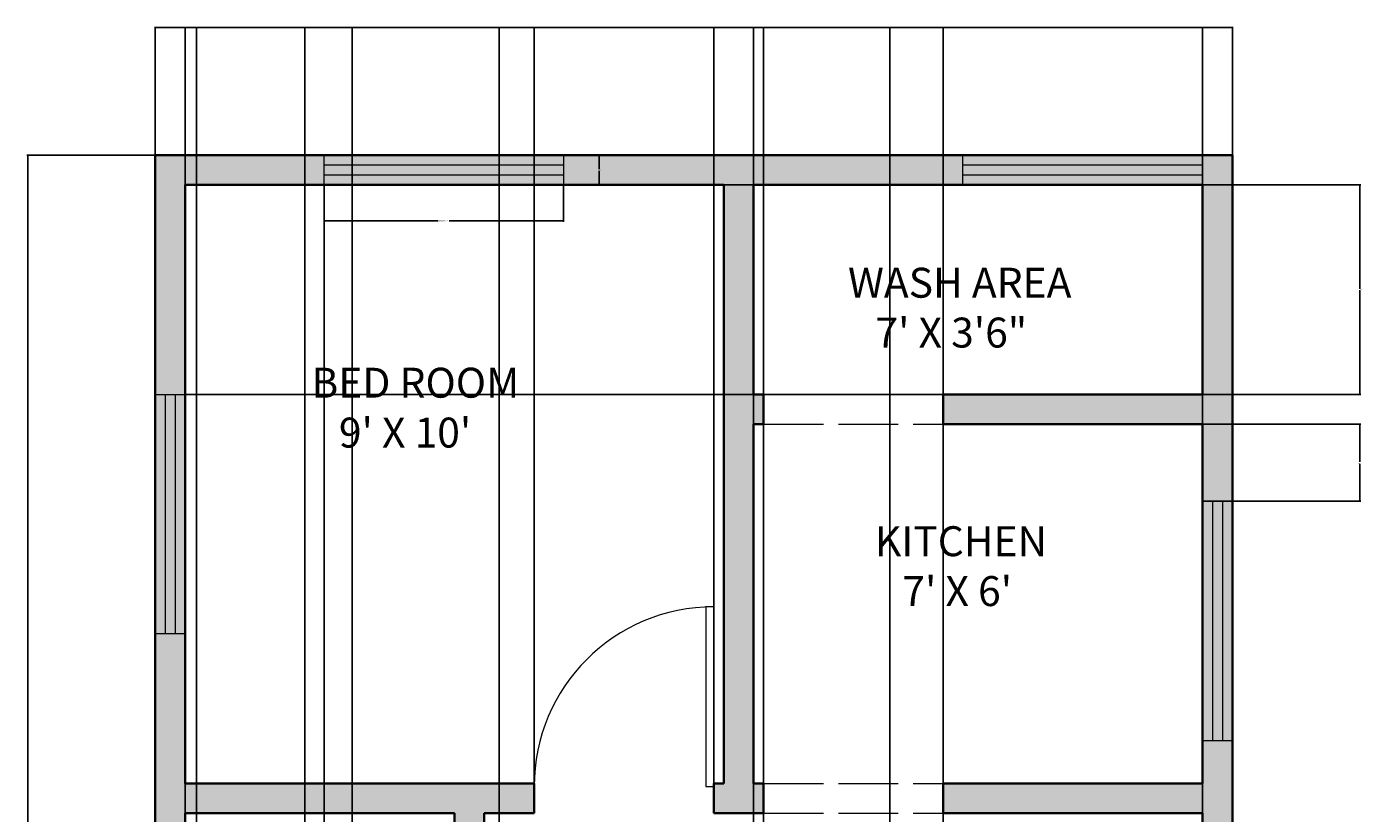
# Model space of a CAD drawing. Units: feet. Extents: x 4596233 to 4596501, y 5666486 to 5667044.
# Tile 3 of 3: x 4596233 to 4596501, y 5666886 to 5667044. Entities that reach past the tile are written whole.
import ezdxf

# ---------------------------------------------------------------- set-up
doc = ezdxf.new("R2010")
doc.units = ezdxf.units.FT
doc.linetypes.add('ACAD_ISO02W100', pattern=[15, 12, -3])
for name, color, linetype, lineweight in [('A-ANNO-DIMS', 2, 'Continuous', 18), ('A-DOOR-OVHD', 240, 'ACAD_ISO02W100', 18), ('A-WALL', 7, 'Continuous', 35), ('ANNOTATION', 170, 'Continuous', 18), ('DOOR', 240, 'Continuous', 18)]:
    doc.layers.add(name, color=color, linetype=linetype, lineweight=lineweight)
doc.layers.add('A-GLAZ', color=2, linetype='Continuous', lineweight=18, true_color=0xf1eb1f)
doc.layers.add('A-WALL-PATT', color=251, linetype='Continuous', lineweight=13, true_color=0x636466)
doc.styles.get("Standard").update_dxf_attribs({"font": 'arial.ttf'})
doc.dimstyles.get("Standard").update_dxf_attribs({"dimtxt": 0.18, "dimasz": 0.18, "dimexe": 0.18, "dimexo": 0.0625, "dimgap": 0.09, "dimtad": 0, "dimtih": 1, "dimtoh": 1, "dimdec": 0, "dimzin": 0, "dimdsep": 46, "dimlunit": 3, "dimtxsty": 'Standard', "dimcen": 0.09, "dimadec": 0, "dimazin": 0, "dimtfac": 1, "dimtdec": 0, "dimtofl": 0, "dimtmove": 0, "dimatfit": 3, "dimfxl": 1, "dimtolj": 1, "dimtzin": 0, "dimarcsym": 0})

# ---------------------------------------------------------------- blocks, each defined once
blk = doc.blocks.new('*U3')
for p, q in [((0, 0), (0, -6)), ((-40, 0), (-40, -6))]:
    blk.add_line(p, q)
blk.add_lwpolyline([(0, 0), (0, 40), (-1.75, 40), (-1.75, 0)], close=True)
blk.add_arc((0, 0), 40, 90, 180)
blk = doc.blocks.new('WIN-48IN')
h = blk.add_hatch(color=256)
h.dxf.hatch_style = 1
h.paths.add_polyline_path([(48, 2), (48, 4), (0, 4), (0, 2)])
for p, q in [((0, 6), (48, 6)), ((0, 0), (0, 6)), ((48, 6), (48, 0)), ((0, 4), (48, 4)), ((0, 2), (48, 2)), ((48, 0), (0, 0))]:
    blk.add_line(p, q)
blk = doc.blocks.new('*D7')
at = {"layer": 'A-ANNO-DIMS', "color": 0, "lineweight": -2, "transparency": 16777216}
for p, q in [((4596292.72, 5667012.09), (4596292.72, 5667004.77)), ((4596340.72, 5667012.09), (4596340.72, 5667004.77)), ((4596292.9, 5667004.95), (4596315.6, 5667004.95)), ((4596340.54, 5667004.95), (4596317.84, 5667004.95))]:
    blk.add_line(p, q, dxfattribs=at)
at = {"layer": 'A-ANNO-DIMS', "color": 0, "transparency": 16777216}
for points in [[(4596292.9, 5667004.98), (4596292.9, 5667004.92), (4596292.72, 5667004.95)], [(4596340.54, 5667004.98), (4596340.54, 5667004.92), (4596340.72, 5667004.95)]]:
    blk.add_solid(points, dxfattribs=at)
at = {"layer": 'Defpoints', "color": 0, "transparency": 16777216}
for p in [(4596292.72, 5667012.15), (4596340.72, 5667012.15), (4596340.72, 5667004.95)]:
    blk.add_point(p, dxfattribs=at)
at = {"layer": 'A-ANNO-DIMS', "color": 0, "transparency": 16777216, "insert": (4596316.72, 5667004.95), "char_height": 0.18, "attachment_point": 5}
blk.add_mtext('\\A1;WINDOW 48 TYP.', dxfattribs=at)
blk = doc.blocks.new('*D8')
at = {"layer": 'A-ANNO-DIMS', "color": 0, "lineweight": -2, "transparency": 16777216}
for p, q in [((4596340.78, 5667018.15), (4596348.1, 5667018.15)), ((4596347.92, 5667017.97), (4596347.92, 5667015.33)), ((4596347.92, 5667012.33), (4596347.92, 5667014.97)), ((4596340.78, 5667012.15), (4596348.1, 5667012.15))]:
    blk.add_line(p, q, dxfattribs=at)
at = {"layer": 'A-ANNO-DIMS', "color": 0, "transparency": 16777216}
for points in [[(4596347.89, 5667017.97), (4596347.95, 5667017.97), (4596347.92, 5667018.15)], [(4596347.89, 5667012.33), (4596347.95, 5667012.33), (4596347.92, 5667012.15)]]:
    blk.add_solid(points, dxfattribs=at)
at = {"layer": 'Defpoints', "color": 0, "transparency": 16777216}
for p in [(4596340.72, 5667018.15), (4596347.92, 5667018.15), (4596340.72, 5667012.15)]:
    blk.add_point(p, dxfattribs=at)
at = {"layer": 'A-ANNO-DIMS', "color": 0, "transparency": 16777216, "insert": (4596347.92, 5667015.15), "char_height": 0.18, "attachment_point": 5}
blk.add_mtext('\\A1;6 TYP.', dxfattribs=at)
blk = doc.blocks.new('*D11')
at = {"layer": 'A-ANNO-DIMS', "color": 0, "lineweight": -2, "transparency": 16777216}
for p, q in [((4596258.85, 5667018.21), (4596258.85, 5667043.88)), ((4596259.03, 5667043.7), (4596366.56, 5667043.7)), ((4596474.67, 5667043.7), (4596367.14, 5667043.7)), ((4596474.85, 5667018.21), (4596474.85, 5667043.88))]:
    blk.add_line(p, q, dxfattribs=at)
at = {"layer": 'A-ANNO-DIMS', "color": 0, "transparency": 16777216}
for points in [[(4596259.03, 5667043.73), (4596259.03, 5667043.67), (4596258.85, 5667043.7)], [(4596474.67, 5667043.73), (4596474.67, 5667043.67), (4596474.85, 5667043.7)]]:
    blk.add_solid(points, dxfattribs=at)
at = {"layer": 'Defpoints', "color": 0, "transparency": 16777216}
for p in [(4596474.85, 5667043.7), (4596258.85, 5667018.15), (4596474.85, 5667018.15)]:
    blk.add_point(p, dxfattribs=at)
at = {"layer": 'A-ANNO-DIMS', "color": 0, "transparency": 16777216, "insert": (4596366.85, 5667043.7), "char_height": 0.18, "attachment_point": 5}
blk.add_mtext('\\A1;216', dxfattribs=at)
blk = doc.blocks.new('*D12')
at = {"layer": 'A-ANNO-DIMS', "color": 0, "lineweight": -2, "transparency": 16777216}
for p, q in [((4596258.79, 5667018.15), (4596233.12, 5667018.15)), ((4596233.3, 5667017.97), (4596233.3, 5666784.33)), ((4596233.3, 5666550.33), (4596233.3, 5666783.97)), ((4596258.79, 5666550.15), (4596233.12, 5666550.15))]:
    blk.add_line(p, q, dxfattribs=at)
at = {"layer": 'A-ANNO-DIMS', "color": 0, "transparency": 16777216}
for points in [[(4596233.27, 5667017.97), (4596233.33, 5667017.97), (4596233.3, 5667018.15)], [(4596233.27, 5666550.33), (4596233.33, 5666550.33), (4596233.3, 5666550.15)]]:
    blk.add_solid(points, dxfattribs=at)
at = {"layer": 'Defpoints', "color": 0, "transparency": 16777216}
for p in [(4596233.3, 5667018.15), (4596258.85, 5667018.15), (4596258.85, 5666550.15)]:
    blk.add_point(p, dxfattribs=at)
at = {"layer": 'A-ANNO-DIMS', "color": 0, "transparency": 16777216, "insert": (4596233.3, 5666784.15), "char_height": 0.18, "attachment_point": 5}
blk.add_mtext('\\A1;468', dxfattribs=at)
blk = doc.blocks.new('*D15')
at = {"layer": 'A-ANNO-DIMS', "color": 0, "lineweight": -2, "transparency": 16777216}
for p, q in [((4596378.85, 5666964.09), (4596378.85, 5666485.84)), ((4596468.85, 5666964.09), (4596468.85, 5666485.84)), ((4596379.03, 5666486.02), (4596423.63, 5666486.02)), ((4596468.67, 5666486.02), (4596424.07, 5666486.02))]:
    blk.add_line(p, q, dxfattribs=at)
at = {"layer": 'A-ANNO-DIMS', "color": 0, "transparency": 16777216}
for points in [[(4596379.03, 5666486.05), (4596379.03, 5666485.99), (4596378.85, 5666486.02)], [(4596468.67, 5666486.05), (4596468.67, 5666485.99), (4596468.85, 5666486.02)]]:
    blk.add_solid(points, dxfattribs=at)
at = {"layer": 'Defpoints', "color": 0, "transparency": 16777216}
for p in [(4596378.85, 5666964.15), (4596468.85, 5666964.15), (4596468.85, 5666486.02)]:
    blk.add_point(p, dxfattribs=at)
at = {"layer": 'A-ANNO-DIMS', "color": 0, "transparency": 16777216, "insert": (4596423.85, 5666486.02), "char_height": 0.18, "attachment_point": 5}
blk.add_mtext('\\A1;90', dxfattribs=at)
blk = doc.blocks.new('*D17')
at = {"layer": 'A-ANNO-DIMS', "color": 0, "lineweight": -2, "transparency": 16777216}
for p, q in [((4596380.85, 5666688.21), (4596380.85, 5667043.88)), ((4596381.03, 5667043.7), (4596398.63, 5667043.7)), ((4596416.67, 5667043.7), (4596399.07, 5667043.7)), ((4596416.85, 5666688.21), (4596416.85, 5667043.88))]:
    blk.add_line(p, q, dxfattribs=at)
at = {"layer": 'A-ANNO-DIMS', "color": 0, "transparency": 16777216}
for points in [[(4596381.03, 5667043.73), (4596381.03, 5667043.67), (4596380.85, 5667043.7)], [(4596416.67, 5667043.73), (4596416.67, 5667043.67), (4596416.85, 5667043.7)]]:
    blk.add_solid(points, dxfattribs=at)
at = {"layer": 'Defpoints', "color": 0, "transparency": 16777216}
for p in [(4596416.85, 5667043.7), (4596380.85, 5666688.15), (4596416.85, 5666688.15)]:
    blk.add_point(p, dxfattribs=at)
at = {"layer": 'A-ANNO-DIMS', "color": 0, "transparency": 16777216, "insert": (4596398.85, 5667043.7), "char_height": 0.18, "attachment_point": 5}
blk.add_mtext('\\A1;36', dxfattribs=at)
blk = doc.blocks.new('*D20')
at = {"layer": 'A-ANNO-DIMS', "color": 0, "lineweight": -2, "transparency": 16777216}
for p, q in [((4596334.85, 5666892.21), (4596334.85, 5667043.88)), ((4596335.03, 5667043.7), (4596352.63, 5667043.7)), ((4596370.67, 5667043.7), (4596353.07, 5667043.7)), ((4596370.85, 5666892.21), (4596370.85, 5667043.88))]:
    blk.add_line(p, q, dxfattribs=at)
at = {"layer": 'A-ANNO-DIMS', "color": 0, "transparency": 16777216}
for points in [[(4596335.03, 5667043.73), (4596335.03, 5667043.67), (4596334.85, 5667043.7)], [(4596370.67, 5667043.73), (4596370.67, 5667043.67), (4596370.85, 5667043.7)]]:
    blk.add_solid(points, dxfattribs=at)
at = {"layer": 'Defpoints', "color": 0, "transparency": 16777216}
for p in [(4596370.85, 5667043.7), (4596334.85, 5666892.15), (4596370.85, 5666892.15)]:
    blk.add_point(p, dxfattribs=at)
at = {"layer": 'A-ANNO-DIMS', "color": 0, "transparency": 16777216, "insert": (4596352.85, 5667043.7), "char_height": 0.18, "attachment_point": 5}
blk.add_mtext('\\A1;36', dxfattribs=at)
blk = doc.blocks.new('*D22')
at = {"layer": 'A-ANNO-DIMS', "color": 0, "lineweight": -2, "transparency": 16777216}
for p, q in [((4596264.85, 5667012.09), (4596264.85, 5666485.84)), ((4596292.72, 5667012.09), (4596292.72, 5666485.84)), ((4596265.03, 5666486.02), (4596278.39, 5666486.02)), ((4596292.54, 5666486.02), (4596279.18, 5666486.02))]:
    blk.add_line(p, q, dxfattribs=at)
at = {"layer": 'A-ANNO-DIMS', "color": 0, "transparency": 16777216}
for points in [[(4596265.03, 5666486.05), (4596265.03, 5666485.99), (4596264.85, 5666486.02)], [(4596292.54, 5666486.05), (4596292.54, 5666485.99), (4596292.72, 5666486.02)]]:
    blk.add_solid(points, dxfattribs=at)
at = {"layer": 'Defpoints', "color": 0, "transparency": 16777216}
for p in [(4596264.85, 5667012.15), (4596292.72, 5667012.15), (4596292.72, 5666486.02)]:
    blk.add_point(p, dxfattribs=at)
at = {"layer": 'A-ANNO-DIMS', "color": 0, "transparency": 16777216, "insert": (4596278.78, 5666486.02), "char_height": 0.18, "attachment_point": 5}
blk.add_mtext('\\A1;27.87', dxfattribs=at)
blk = doc.blocks.new('*D23')
at = {"layer": 'A-ANNO-DIMS', "color": 0, "lineweight": -2, "transparency": 16777216}
for p, q in [((4596264.91, 5667012.15), (4596500.58, 5667012.15)), ((4596500.4, 5667011.97), (4596500.4, 5666991.32)), ((4596500.4, 5666970.3), (4596500.4, 5666990.95)), ((4596264.91, 5666970.12), (4596500.58, 5666970.12))]:
    blk.add_line(p, q, dxfattribs=at)
at = {"layer": 'A-ANNO-DIMS', "color": 0, "transparency": 16777216}
for points in [[(4596500.37, 5667011.97), (4596500.43, 5667011.97), (4596500.4, 5667012.15)], [(4596500.37, 5666970.3), (4596500.43, 5666970.3), (4596500.4, 5666970.12)]]:
    blk.add_solid(points, dxfattribs=at)
at = {"layer": 'Defpoints', "color": 0, "transparency": 16777216}
for p in [(4596264.85, 5667012.15), (4596500.4, 5667012.15), (4596264.85, 5666970.12)]:
    blk.add_point(p, dxfattribs=at)
at = {"layer": 'A-ANNO-DIMS', "color": 0, "transparency": 16777216, "insert": (4596500.4, 5666991.13), "char_height": 0.18, "attachment_point": 5}
blk.add_mtext('\\A1;42.03', dxfattribs=at)
blk = doc.blocks.new('*D24')
at = {"layer": 'A-ANNO-DIMS', "color": 0, "lineweight": -2, "transparency": 16777216}
for p, q in [((4596468.91, 5666964.15), (4596500.58, 5666964.15)), ((4596500.4, 5666963.97), (4596500.4, 5666956.61)), ((4596500.4, 5666948.89), (4596500.4, 5666956.25)), ((4596468.91, 5666948.71), (4596500.58, 5666948.71))]:
    blk.add_line(p, q, dxfattribs=at)
at = {"layer": 'A-ANNO-DIMS', "color": 0, "transparency": 16777216}
for points in [[(4596500.37, 5666963.97), (4596500.43, 5666963.97), (4596500.4, 5666964.15)], [(4596500.37, 5666948.89), (4596500.43, 5666948.89), (4596500.4, 5666948.71)]]:
    blk.add_solid(points, dxfattribs=at)
at = {"layer": 'Defpoints', "color": 0, "transparency": 16777216}
for p in [(4596468.85, 5666964.15), (4596468.85, 5666948.71), (4596500.4, 5666948.71)]:
    blk.add_point(p, dxfattribs=at)
at = {"layer": 'A-ANNO-DIMS', "color": 0, "transparency": 16777216, "insert": (4596500.4, 5666956.43), "char_height": 0.18, "attachment_point": 5}
blk.add_mtext('\\A1;15.44', dxfattribs=at)
blk = doc.blocks.new('*D28')
at = {"layer": 'A-ANNO-DIMS', "color": 0, "lineweight": -2, "transparency": 16777216}
for p, q in [((4596378.85, 5666556.21), (4596378.85, 5667043.88)), ((4596379.03, 5667043.7), (4596392.04, 5667043.7)), ((4596405.99, 5667043.7), (4596392.97, 5667043.7)), ((4596406.17, 5666556.21), (4596406.17, 5667043.88))]:
    blk.add_line(p, q, dxfattribs=at)
at = {"layer": 'A-ANNO-DIMS', "color": 0, "transparency": 16777216}
for points in [[(4596379.03, 5667043.73), (4596379.03, 5667043.67), (4596378.85, 5667043.7)], [(4596405.99, 5667043.73), (4596405.99, 5667043.67), (4596406.17, 5667043.7)]]:
    blk.add_solid(points, dxfattribs=at)
at = {"layer": 'Defpoints', "color": 0, "transparency": 16777216}
for p in [(4596406.17, 5667043.7), (4596378.85, 5666556.15), (4596406.17, 5666556.15)]:
    blk.add_point(p, dxfattribs=at)
at = {"layer": 'A-ANNO-DIMS', "color": 0, "transparency": 16777216, "insert": (4596392.51, 5667043.7), "char_height": 0.18, "attachment_point": 5}
blk.add_mtext('\\A1;27.317', dxfattribs=at)
blk = doc.blocks.new('*D33')
at = {"layer": 'A-ANNO-DIMS', "color": 0, "lineweight": -2, "transparency": 16777216}
for p, q in [((4596267.15, 5666650.02), (4596267.15, 5667043.88)), ((4596267.33, 5667043.7), (4596282.36, 5667043.7)), ((4596298.17, 5667043.7), (4596283.14, 5667043.7)), ((4596298.35, 5666650.02), (4596298.35, 5667043.88))]:
    blk.add_line(p, q, dxfattribs=at)
at = {"layer": 'A-ANNO-DIMS', "color": 0, "transparency": 16777216}
for points in [[(4596267.33, 5667043.73), (4596267.33, 5667043.67), (4596267.15, 5667043.7)], [(4596298.17, 5667043.73), (4596298.17, 5667043.67), (4596298.35, 5667043.7)]]:
    blk.add_solid(points, dxfattribs=at)
at = {"layer": 'Defpoints', "color": 0, "transparency": 16777216}
for p in [(4596298.35, 5667043.7), (4596267.15, 5666649.96), (4596298.35, 5666649.96)]:
    blk.add_point(p, dxfattribs=at)
at = {"layer": 'A-ANNO-DIMS', "color": 0, "transparency": 16777216, "insert": (4596282.75, 5667043.7), "char_height": 0.18, "attachment_point": 5}
blk.add_mtext('\\A1;31.19', dxfattribs=at)
blk = doc.blocks.new('*D34')
at = {"layer": 'A-ANNO-DIMS', "color": 0, "lineweight": -2, "transparency": 16777216}
for p, q in [((4596264.85, 5666892.21), (4596264.85, 5667043.88)), ((4596265.03, 5667043.7), (4596299.63, 5667043.7)), ((4596334.67, 5667043.7), (4596300.07, 5667043.7)), ((4596334.85, 5666892.21), (4596334.85, 5667043.88))]:
    blk.add_line(p, q, dxfattribs=at)
at = {"layer": 'A-ANNO-DIMS', "color": 0, "transparency": 16777216}
for points in [[(4596265.03, 5667043.73), (4596265.03, 5667043.67), (4596264.85, 5667043.7)], [(4596334.67, 5667043.73), (4596334.67, 5667043.67), (4596334.85, 5667043.7)]]:
    blk.add_solid(points, dxfattribs=at)
at = {"layer": 'Defpoints', "color": 0, "transparency": 16777216}
for p in [(4596334.85, 5667043.7), (4596264.85, 5666892.15), (4596334.85, 5666892.15)]:
    blk.add_point(p, dxfattribs=at)
at = {"layer": 'A-ANNO-DIMS', "color": 0, "transparency": 16777216, "insert": (4596299.85, 5667043.7), "char_height": 0.18, "attachment_point": 5}
blk.add_mtext('\\A1;70', dxfattribs=at)
blk = doc.blocks.new('*D35')
at = {"layer": 'A-ANNO-DIMS', "color": 0, "lineweight": -2, "transparency": 16777216}
for p, q in [((4596416.85, 5666688.21), (4596416.85, 5667043.88)), ((4596417.03, 5667043.7), (4596442.63, 5667043.7)), ((4596468.67, 5667043.7), (4596443.07, 5667043.7)), ((4596468.85, 5666688.21), (4596468.85, 5667043.88))]:
    blk.add_line(p, q, dxfattribs=at)
at = {"layer": 'A-ANNO-DIMS', "color": 0, "transparency": 16777216}
for points in [[(4596417.03, 5667043.73), (4596417.03, 5667043.67), (4596416.85, 5667043.7)], [(4596468.67, 5667043.73), (4596468.67, 5667043.67), (4596468.85, 5667043.7)]]:
    blk.add_solid(points, dxfattribs=at)
at = {"layer": 'Defpoints', "color": 0, "transparency": 16777216}
for p in [(4596468.85, 5667043.7), (4596416.85, 5666688.15), (4596468.85, 5666688.15)]:
    blk.add_point(p, dxfattribs=at)
at = {"layer": 'A-ANNO-DIMS', "color": 0, "transparency": 16777216, "insert": (4596442.85, 5667043.7), "char_height": 0.18, "attachment_point": 5}
blk.add_mtext('\\A1;52', dxfattribs=at)
blk = doc.blocks.new('*D37')
at = {"layer": 'A-ANNO-DIMS', "color": 0, "lineweight": -2, "transparency": 16777216}
for p, q in [((4596264.85, 5666688.21), (4596264.85, 5667043.88)), ((4596265.03, 5667043.7), (4596296.13, 5667043.7)), ((4596327.67, 5667043.7), (4596296.57, 5667043.7)), ((4596327.85, 5666688.21), (4596327.85, 5667043.88))]:
    blk.add_line(p, q, dxfattribs=at)
at = {"layer": 'A-ANNO-DIMS', "color": 0, "transparency": 16777216}
for points in [[(4596265.03, 5667043.73), (4596265.03, 5667043.67), (4596264.85, 5667043.7)], [(4596327.67, 5667043.73), (4596327.67, 5667043.67), (4596327.85, 5667043.7)]]:
    blk.add_solid(points, dxfattribs=at)
at = {"layer": 'Defpoints', "color": 0, "transparency": 16777216}
for p in [(4596327.85, 5667043.7), (4596264.85, 5666688.15), (4596327.85, 5666688.15)]:
    blk.add_point(p, dxfattribs=at)
at = {"layer": 'A-ANNO-DIMS', "color": 0, "transparency": 16777216, "insert": (4596296.35, 5667043.7), "char_height": 0.18, "attachment_point": 5}
blk.add_mtext('\\A1;63', dxfattribs=at)
blk = doc.blocks.new('*D39')
at = {"layer": 'A-ANNO-DIMS', "color": 0, "lineweight": -2, "transparency": 16777216}
for p, q in [((4596264.85, 5666760.21), (4596264.85, 5667043.88)), ((4596265.03, 5667043.7), (4596276.63, 5667043.7)), ((4596288.67, 5667043.7), (4596277.07, 5667043.7)), ((4596288.85, 5666760.21), (4596288.85, 5667043.88))]:
    blk.add_line(p, q, dxfattribs=at)
at = {"layer": 'A-ANNO-DIMS', "color": 0, "transparency": 16777216}
for points in [[(4596265.03, 5667043.73), (4596265.03, 5667043.67), (4596264.85, 5667043.7)], [(4596288.67, 5667043.73), (4596288.67, 5667043.67), (4596288.85, 5667043.7)]]:
    blk.add_solid(points, dxfattribs=at)
at = {"layer": 'Defpoints', "color": 0, "transparency": 16777216}
for p in [(4596288.85, 5667043.7), (4596264.85, 5666760.15), (4596288.85, 5666760.15)]:
    blk.add_point(p, dxfattribs=at)
at = {"layer": 'A-ANNO-DIMS', "color": 0, "transparency": 16777216, "insert": (4596276.85, 5667043.7), "char_height": 0.18, "attachment_point": 5}
blk.add_mtext('\\A1;24', dxfattribs=at)
blk = doc.blocks.new('*D43')
at = {"layer": 'A-ANNO-DIMS', "color": 0, "lineweight": -2, "transparency": 16777216}
for p, q in [((4596380.85, 5666970.21), (4596380.85, 5667043.88)), ((4596381.03, 5667043.7), (4596398.63, 5667043.7)), ((4596416.67, 5667043.7), (4596399.07, 5667043.7)), ((4596416.85, 5666970.21), (4596416.85, 5667043.88))]:
    blk.add_line(p, q, dxfattribs=at)
at = {"layer": 'A-ANNO-DIMS', "color": 0, "transparency": 16777216}
for points in [[(4596381.03, 5667043.73), (4596381.03, 5667043.67), (4596380.85, 5667043.7)], [(4596416.67, 5667043.73), (4596416.67, 5667043.67), (4596416.85, 5667043.7)]]:
    blk.add_solid(points, dxfattribs=at)
at = {"layer": 'Defpoints', "color": 0, "transparency": 16777216}
for p in [(4596416.85, 5667043.7), (4596380.85, 5666970.15), (4596416.85, 5666970.15)]:
    blk.add_point(p, dxfattribs=at)
at = {"layer": 'A-ANNO-DIMS', "color": 0, "transparency": 16777216, "insert": (4596398.85, 5667043.7), "char_height": 0.18, "attachment_point": 5}
blk.add_mtext('\\A1;36', dxfattribs=at)

msp = doc.modelspace()

# ---------------------------------------------------------------- hatches: boundary and pattern name
at = {"layer": 'A-WALL-PATT'}
h = msp.add_hatch(color=256, dxfattribs=at)
h.dxf.hatch_style = 1
h.paths.add_polyline_path([(4596474.8511, 5667018.1479), (4596258.8511, 5667018.1479), (4596258.8511, 5666550.1479), (4596474.8511, 5666550.1479)])
h.paths.add_polyline_path([(4596372.8511, 5667012.1479), (4596372.8511, 5666892.1479), (4596370.8511, 5666892.1479), (4596370.8511, 5666891.5479), (4596370.8511, 5666886.1479), (4596380.8511, 5666886.1479), (4596380.8511, 5666892.1479), (4596378.8511, 5666892.1479), (4596378.8511, 5666964.1479), (4596380.8511, 5666964.1479), (4596380.8511, 5666970.1479), (4596378.8511, 5666970.1479), (4596378.8511, 5667012.1479), (4596468.8511, 5667012.1479), (4596468.8511, 5666970.1479), (4596416.8511, 5666970.1479), (4596416.8511, 5666964.1479), (4596468.8511, 5666964.1479), (4596468.8511, 5666892.1479), (4596416.8511, 5666892.1479), (4596416.8511, 5666886.1479), (4596468.8511, 5666886.1479), (4596468.8511, 5666688.1479), (4596416.8511, 5666688.1479), (4596416.8511, 5666682.1479), (4596468.8511, 5666682.1479), (4596468.8511, 5666556.1479), (4596378.8511, 5666556.1479), (4596378.8511, 5666682.1479), (4596380.8511, 5666682.1479), (4596380.8511, 5666687.5479), (4596380.8511, 5666688.1479), (4596369.8511, 5666688.1479), (4596369.8511, 5666685.2979), (4596369.8511, 5666682.1479), (4596372.8511, 5666682.1479), (4596372.8511, 5666556.1479), (4596264.8511, 5666556.1479), (4596264.8511, 5666682.1479), (4596327.8511, 5666682.1479), (4596327.8511, 5666685.2979), (4596327.8511, 5666688.1479), (4596324.8511, 5666688.1479), (4596324.8511, 5666772.1479), (4596318.8511, 5666772.1479), (4596318.8511, 5666760.1479), (4596318.8511, 5666754.1479), (4596318.8511, 5666724.1479), (4596318.8511, 5666688.1479), (4596264.8511, 5666688.1479), (4596264.8511, 5666754.1479), (4596288.8511, 5666754.1479), (4596288.8511, 5666758.6479), (4596288.8511, 5666760.1479), (4596264.8511, 5666760.1479), (4596264.8511, 5666814.1479), (4596288.8511, 5666814.1479), (4596288.8511, 5666818.6479), (4596288.8511, 5666820.1479), (4596264.8511, 5666820.1479), (4596264.8511, 5666886.1479), (4596318.8511, 5666886.1479), (4596318.8511, 5666820.1479), (4596318.8511, 5666818.6479), (4596318.8511, 5666814.1479), (4596318.8511, 5666802.1479), (4596324.8511, 5666802.1479), (4596324.8511, 5666886.1479), (4596334.8511, 5666886.1479), (4596334.8511, 5666891.5479), (4596334.8511, 5666892.1479), (4596264.8511, 5666892.1479), (4596264.8511, 5667012.1479)], flags=16)
h.paths.add_polyline_path([(4596316.6338, 5666680.1479), (4596316.6338, 5666661.9608), (4596301.036, 5666661.9608), (4596301.036, 5666589.119), (4596370.916, 5666589.119), (4596370.916, 5666558.119), (4596267.1547, 5666558.119), (4596267.1547, 5666680.1479)], flags=0)
h.paths.add_polyline_path([(4596282.7503, 5666649.9608), (4596298.3459, 5666649.9608), (4596298.3459, 5666586.4128), (4596333.2108, 5666586.4128), (4596333.2108, 5666572.6335), (4596282.7503, 5666572.6335)], flags=0)
h.paths.add_polyline_path([(4596380.8511, 5666682.1479), (4596382.4261, 5666682.1479), (4596382.4261, 5666646.1479), (4596380.8511, 5666646.1479)], flags=0)
h.paths.add_polyline_path([(4596270.4341, 5666856.9819), (4596311.4805, 5666856.9819), (4596311.4805, 5666879.3708), (4596270.4341, 5666879.3708)], flags=8)
h.paths.add_polyline_path([(4596271.3283, 5666778.1649), (4596312.3747, 5666778.1649), (4596312.3747, 5666800.5538), (4596271.3283, 5666800.5538)], flags=8)
h.paths.add_polyline_path([(4596401.0723, 5666924.3036), (4596440.8622, 5666924.3036), (4596440.8622, 5666946.6925), (4596401.0723, 5666946.6925)], flags=8)
h.paths.add_polyline_path([(4596396.1839, 5666976.1395), (4596449.4963, 5666976.1395), (4596449.4963, 5666998.5283), (4596396.1839, 5666998.5283)], flags=8)
h.paths.add_polyline_path([(4596288.0879, 5666956.0844), (4596336.7264, 5666956.0844), (4596336.7264, 5666978.4732), (4596288.0879, 5666978.4732)], flags=8)
h.paths.add_polyline_path([(4596267.7433, 5666702.4027), (4596308.7897, 5666702.4027), (4596308.7897, 5666724.7916), (4596267.7433, 5666724.7916)], flags=8)
h.paths.add_polyline_path([(4596371.4978, 5666770.3665), (4596425.2768, 5666770.3665), (4596425.2768, 5666792.7553), (4596371.4978, 5666792.7553)], flags=8)
h.paths.add_polyline_path([(4596414.2198, 5666615.8536), (4596452.2908, 5666615.8536), (4596452.2908, 5666638.2424), (4596414.2198, 5666638.2424)], flags=8)
h.paths.add_polyline_path([(4596310.1554, 5666620.3865), (4596350.8825, 5666620.3865), (4596350.8825, 5666642.7753), (4596310.1554, 5666642.7753)], flags=8)
h = msp.add_hatch(color=256, dxfattribs=at)
h.dxf.hatch_style = 1
h.paths.add_polyline_path([(4596474.8511, 5667018.1479), (4596258.8511, 5667018.1479), (4596258.8511, 5666550.1479), (4596474.8511, 5666550.1479)])
h.paths.add_polyline_path([(4596468.8511, 5666970.1479), (4596416.8511, 5666970.1479), (4596416.8511, 5666964.1479), (4596468.8511, 5666964.1479), (4596468.8511, 5666892.1479), (4596416.8511, 5666892.1479), (4596416.8511, 5666886.1479), (4596468.8511, 5666886.1479), (4596468.8511, 5666688.1479), (4596416.8511, 5666688.1479), (4596416.8511, 5666682.1479), (4596468.8511, 5666682.1479), (4596468.8511, 5666556.1479), (4596378.8511, 5666556.1479), (4596378.8511, 5666682.1479), (4596380.8511, 5666682.1479), (4596380.8511, 5666687.5479), (4596380.8511, 5666688.1479), (4596369.8511, 5666688.1479), (4596369.8511, 5666685.2979), (4596369.8511, 5666682.1479), (4596372.8511, 5666682.1479), (4596372.8511, 5666556.1479), (4596264.8511, 5666556.1479), (4596264.8511, 5666682.1479), (4596327.8511, 5666682.1479), (4596327.8511, 5666685.2979), (4596327.8511, 5666688.1479), (4596324.8511, 5666688.1479), (4596324.8511, 5666772.1479), (4596318.8511, 5666772.1479), (4596318.8511, 5666760.1479), (4596318.8511, 5666754.1479), (4596318.8511, 5666724.1479), (4596318.8511, 5666688.1479), (4596264.8511, 5666688.1479), (4596264.8511, 5666754.1479), (4596288.8511, 5666754.1479), (4596288.8511, 5666758.6479), (4596288.8511, 5666760.1479), (4596264.8511, 5666760.1479), (4596264.8511, 5666814.1479), (4596288.8511, 5666814.1479), (4596288.8511, 5666818.6479), (4596288.8511, 5666820.1479), (4596264.8511, 5666820.1479), (4596264.8511, 5666886.1479), (4596318.8511, 5666886.1479), (4596318.8511, 5666820.1479), (4596318.8511, 5666818.6479), (4596318.8511, 5666814.1479), (4596318.8511, 5666802.1479), (4596324.8511, 5666802.1479), (4596324.8511, 5666886.1479), (4596334.8511, 5666886.1479), (4596334.8511, 5666891.5479), (4596334.8511, 5666892.1479), (4596264.8511, 5666892.1479), (4596264.8511, 5667012.1479), (4596372.8511, 5667012.1479), (4596372.8511, 5666892.1479), (4596370.8511, 5666892.1479), (4596370.8511, 5666891.5479), (4596370.8511, 5666886.1479), (4596380.8511, 5666886.1479), (4596380.8511, 5666892.1479), (4596378.8511, 5666892.1479), (4596378.8511, 5666964.1479), (4596380.8511, 5666964.1479), (4596380.8511, 5666970.1479), (4596378.8511, 5666970.1479), (4596378.8511, 5667012.1479), (4596468.8511, 5667012.1479)], flags=16)
h.paths.add_polyline_path([(4596382.4261, 5666646.1479), (4596380.8511, 5666646.1479), (4596380.8511, 5666682.1479), (4596382.4261, 5666682.1479)], flags=0)
h.paths.add_polyline_path([(4596316.6338, 5666680.1479), (4596316.6338, 5666661.9608), (4596301.036, 5666661.9608), (4596301.036, 5666589.119), (4596370.916, 5666589.119), (4596370.916, 5666558.119), (4596267.1547, 5666558.119), (4596267.1547, 5666680.1479)], flags=0)
h.paths.add_polyline_path([(4596282.7503, 5666649.9608), (4596298.3459, 5666649.9608), (4596298.3459, 5666586.4128), (4596333.2108, 5666586.4128), (4596333.2108, 5666572.6335), (4596282.7503, 5666572.6335)], flags=0)
h.paths.add_polyline_path([(4596270.4341, 5666856.9819), (4596311.4805, 5666856.9819), (4596311.4805, 5666879.3708), (4596270.4341, 5666879.3708)], flags=8)
h.paths.add_polyline_path([(4596271.3283, 5666778.1649), (4596312.3747, 5666778.1649), (4596312.3747, 5666800.5538), (4596271.3283, 5666800.5538)], flags=8)
h.paths.add_polyline_path([(4596401.0723, 5666924.3036), (4596440.8622, 5666924.3036), (4596440.8622, 5666946.6925), (4596401.0723, 5666946.6925)], flags=8)
h.paths.add_polyline_path([(4596396.1839, 5666976.1395), (4596449.4963, 5666976.1395), (4596449.4963, 5666998.5283), (4596396.1839, 5666998.5283)], flags=8)
h.paths.add_polyline_path([(4596288.0879, 5666956.0844), (4596336.7264, 5666956.0844), (4596336.7264, 5666978.4732), (4596288.0879, 5666978.4732)], flags=8)
h.paths.add_polyline_path([(4596267.7433, 5666702.4027), (4596308.7897, 5666702.4027), (4596308.7897, 5666724.7916), (4596267.7433, 5666724.7916)], flags=8)
h.paths.add_polyline_path([(4596371.4978, 5666770.3665), (4596425.2768, 5666770.3665), (4596425.2768, 5666792.7553), (4596371.4978, 5666792.7553)], flags=8)
h.paths.add_polyline_path([(4596414.2198, 5666615.8536), (4596452.2908, 5666615.8536), (4596452.2908, 5666638.2424), (4596414.2198, 5666638.2424)], flags=8)
h.paths.add_polyline_path([(4596310.1554, 5666620.3865), (4596350.8825, 5666620.3865), (4596350.8825, 5666642.7753), (4596310.1554, 5666642.7753)], flags=8)

# ---------------------------------------------------------------- linework, layer by layer
at = {"layer": 'A-DOOR-OVHD'}
for p, q in [((4596380.8511, 5666970.1479), (4596416.8511, 5666970.1479)), ((4596380.8511, 5666964.1479), (4596416.8511, 5666964.1479)), ((4596380.8511, 5666892.1479), (4596416.8511, 5666892.1479)), ((4596380.8511, 5666886.1479), (4596416.8511, 5666886.1479))]:
    msp.add_line(p, q, dxfattribs=at)
at = {"layer": 'A-WALL'}
for p, q in [((4596258.8511, 5667018.1479), (4596474.8511, 5667018.1479)), ((4596258.8511, 5666550.1479), (4596258.8511, 5667018.1479)), ((4596474.8511, 5667018.1479), (4596474.8511, 5666550.1479)), ((4596264.8511, 5667012.1479), (4596372.8511, 5667012.1479)), ((4596264.8511, 5666892.1479), (4596264.8511, 5667012.1479)), ((4596372.8511, 5666892.1479), (4596372.8511, 5667012.1479)), ((4596378.8511, 5667012.1479), (4596468.8511, 5667012.1479)), ((4596378.8511, 5666970.1479), (4596378.8511, 5667012.1479)), ((4596468.8511, 5667012.1479), (4596468.8511, 5666970.1479)), ((4596378.8511, 5666970.1479), (4596380.8511, 5666970.1479)), ((4596380.8511, 5666970.1479), (4596380.8511, 5666964.1479)), ((4596416.8511, 5666970.1479), (4596416.8511, 5666964.1479)), ((4596416.8511, 5666970.1479), (4596468.8511, 5666970.1479)), ((4596378.8511, 5666964.1479), (4596380.8511, 5666964.1479)), ((4596378.8511, 5666892.1479), (4596378.8511, 5666964.1479)), ((4596416.8511, 5666964.1479), (4596468.8511, 5666964.1479)), ((4596468.8511, 5666964.1479), (4596468.8511, 5666892.1479)), ((4596264.8511, 5666892.1479), (4596334.8511, 5666892.1479)), ((4596334.8511, 5666892.1479), (4596334.8511, 5666886.1479)), ((4596370.8511, 5666892.1479), (4596370.8511, 5666886.1479)), ((4596370.8511, 5666892.1479), (4596372.8511, 5666892.1479)), ((4596378.8511, 5666892.1479), (4596380.8511, 5666892.1479)), ((4596380.8511, 5666892.1479), (4596380.8511, 5666886.1479)), ((4596416.8511, 5666892.1479), (4596416.8511, 5666886.1479)), ((4596416.8511, 5666892.1479), (4596468.8511, 5666892.1479)), ((4596264.8511, 5666886.1479), (4596318.8511, 5666886.1479)), ((4596264.8511, 5666820.1479), (4596264.8511, 5666886.1479)), ((4596318.8511, 5666820.1479), (4596318.8511, 5666886.1479)), ((4596324.8511, 5666886.1479), (4596334.8511, 5666886.1479)), ((4596324.8511, 5666802.1479), (4596324.8511, 5666886.1479)), ((4596370.8511, 5666886.1479), (4596380.8511, 5666886.1479)), ((4596416.8511, 5666886.1479), (4596468.8511, 5666886.1479)), ((4596468.8511, 5666886.1479), (4596468.8511, 5666688.1479))]:
    msp.add_line(p, q, dxfattribs=at)

# ---------------------------------------------------------------- block references
at = {"layer": 'A-GLAZ'}
for p in [(4596292.718, 5667012.148), (4596420.7753, 5667012.148)]:
    msp.add_blockref('WIN-48IN', p, dxfattribs=at)
for p, rotation in [((4596258.8512, 5666970.1206), 270.0000000038905), ((4596468.8512, 5666948.707), 270.0000000067078)]:
    msp.add_blockref('WIN-48IN', p, dxfattribs=dict(at, rotation=rotation))
at = {"layer": 'DOOR', "xscale": 0.9000000000838191, "yscale": 0.9000000000838191, "zscale": 0.9000000000838191}
msp.add_blockref('*U3', (4596370.8511, 5666891.5479), dxfattribs=at)

# ---------------------------------------------------------------- texts
at = {"layer": 'ANNOTATION', "char_height": 6, "attachment_point": 1}
for s, width, insert in [('WASH AREA\\P   7\' X 3\'6"', 50.67683, (4596397.7863, 5666995.5427)), ("BED ROOM\\P   9' X 10'", 52.338365, (4596290.2018, 5666975.4916)), ("KITCHEN\\P   7' X 6'", 41.538385, (4596403.1862, 5666943.7068))]:
    msp.add_mtext_dynamic_manual_height_columns(s, width=width, gutter_width=12.5, heights=[0], dxfattribs=dict(at, insert=insert))

# ---------------------------------------------------------------- dimensions: what is measured, and where the dimension line sits
at = {"layer": 'A-ANNO-DIMS'}
for base, p1, p2, override, picture, middle in [((4596474.8511, 5667043.6979), (4596258.8511, 5667018.1479), (4596474.8511, 5667018.1479), {"dimdec": 0, "dimlfac": 1, "dimrnd": 0, "dimzin": 0, "dimdsep": 46, "dimlunit": 2}, '*D11', (4596366.8511, 5667043.6979)), ((4596334.8511, 5667043.6979), (4596264.8511, 5666892.1479), (4596334.8511, 5666892.1479), {"dimdec": 0, "dimlfac": 1, "dimrnd": 0, "dimzin": 0, "dimdsep": 46, "dimlunit": 2}, '*D34', (4596299.8511, 5667043.6979)), ((4596327.8511, 5667043.6979), (4596264.8511, 5666688.1479), (4596327.8511, 5666688.1479), {"dimdec": 0, "dimlfac": 1, "dimrnd": 0, "dimzin": 0, "dimdsep": 46, "dimlunit": 2}, '*D37', (4596296.3511, 5667043.6979)), ((4596288.8511, 5667043.6979), (4596264.8511, 5666760.1479), (4596288.8511, 5666760.1479), {"dimdec": 0, "dimlfac": 1, "dimrnd": 0, "dimzin": 0, "dimdsep": 46, "dimlunit": 2}, '*D39', (4596276.8511, 5667043.6979)), ((4596298.3459, 5667043.6979), (4596267.1547, 5666649.9608), (4596298.3459, 5666649.9608), {"dimdec": 2, "dimlfac": 1, "dimrnd": 0, "dimzin": 0, "dimdsep": 46, "dimlunit": 2}, '*D33', (4596282.7503, 5667043.6979)), ((4596370.8511, 5667043.6979), (4596334.8511, 5666892.1479), (4596370.8511, 5666892.1479), {"dimdec": 0, "dimlfac": 1, "dimrnd": 0, "dimzin": 0, "dimdsep": 46, "dimlunit": 2}, '*D20', (4596352.8511, 5667043.6979)), ((4596406.1677, 5667043.6979), (4596378.8511, 5666556.1479), (4596406.1677, 5666556.1479), {"dimdec": 3, "dimlfac": 1, "dimrnd": 0, "dimzin": 0, "dimdsep": 46, "dimlunit": 2}, '*D28', (4596392.5094, 5667043.6979)), ((4596416.8511, 5667043.6979), (4596380.8511, 5666688.1479), (4596416.8511, 5666688.1479), {"dimdec": 0, "dimlfac": 1, "dimrnd": 0, "dimzin": 0, "dimdsep": 46, "dimlunit": 2}, '*D17', (4596398.8511, 5667043.6979)), ((4596416.8511, 5667043.6979), (4596380.8511, 5666970.1479), (4596416.8511, 5666970.1479), {"dimdec": 0, "dimlfac": 1, "dimrnd": 0, "dimzin": 0, "dimdsep": 46, "dimlunit": 2}, '*D43', (4596398.8511, 5667043.6979)), ((4596468.8511, 5667043.6979), (4596416.8511, 5666688.1479), (4596468.8511, 5666688.1479), {"dimdec": 0, "dimlfac": 1, "dimrnd": 0, "dimzin": 0, "dimdsep": 46, "dimlunit": 2}, '*D35', (4596442.8511, 5667043.6979)), ((4596292.7184, 5666486.0229), (4596264.8511, 5667012.1479), (4596292.7184, 5667012.1479), {"dimdec": 2, "dimlfac": 1, "dimrnd": 0, "dimzin": 0, "dimdsep": 46, "dimlunit": 2}, '*D22', (4596278.7847, 5666486.0229)), ((4596468.8511, 5666486.0229), (4596378.8511, 5666964.1479), (4596468.8511, 5666964.1479), {"dimdec": 0, "dimlfac": 1, "dimrnd": 0, "dimzin": 0, "dimdsep": 46, "dimlunit": 2}, '*D15', (4596423.8511, 5666486.0229))]:
    dim = msp.add_linear_dim(base=base, p1=p1, p2=p2, dimstyle='Standard', override=override, dxfattribs=at)
    dim.commit()
    dim.dimension.update_dxf_attribs({"geometry": picture, "text_midpoint": middle})
for base, p1, p2, override, picture, middle in [((4596233.3011, 5667018.1479), (4596258.8511, 5666550.1479), (4596258.8511, 5667018.1479), {"dimdec": 0, "dimlfac": 1, "dimrnd": 0, "dimzin": 0, "dimdsep": 46, "dimlunit": 2}, '*D12', (4596233.3011, 5666784.1479)), ((4596500.4011, 5667012.1479), (4596264.8511, 5666970.1202), (4596264.8511, 5667012.1479), {"dimdec": 2, "dimlfac": 1, "dimrnd": 0, "dimzin": 0, "dimdsep": 46, "dimlunit": 2}, '*D23', (4596500.4011, 5666991.1341)), ((4596500.4011, 5666948.7066), (4596468.8511, 5666964.1479), (4596468.8511, 5666948.7066), {"dimdec": 2, "dimlfac": 1, "dimrnd": 0, "dimzin": 0, "dimdsep": 46, "dimlunit": 2}, '*D24', (4596500.4011, 5666956.4273))]:
    dim = msp.add_linear_dim(base=base, p1=p1, p2=p2, angle=90, dimstyle='Standard', override=override, dxfattribs=at)
    dim.commit()
    dim.dimension.update_dxf_attribs({"geometry": picture, "text_midpoint": middle})
dim = msp.add_linear_dim(base=(4596347.9184, 5667018.1479), p1=(4596340.7184, 5667012.1479), p2=(4596340.7184, 5667018.1479), angle=90, text='<> TYP.', dimstyle='Standard', override={"dimdec": 0, "dimlfac": 1, "dimrnd": 0, "dimzin": 0, "dimdsep": 46, "dimlunit": 2}, dxfattribs=at)
dim.commit()
dim.dimension.update_dxf_attribs({"geometry": '*D8', "text_midpoint": (4596347.9184, 5667015.1479)})
dim = msp.add_linear_dim(base=(4596340.7184, 5667004.9479), p1=(4596292.7184, 5667012.1479), p2=(4596340.7184, 5667012.1479), text='WINDOW <> TYP.', dimstyle='Standard', override={"dimdec": 0, "dimlfac": 1, "dimrnd": 0, "dimzin": 0, "dimdsep": 46, "dimlunit": 2}, dxfattribs=at)
dim.commit()
dim.dimension.update_dxf_attribs({"geometry": '*D7', "text_midpoint": (4596316.7184, 5667004.9479)})

doc.saveas('drawing.dxf')
